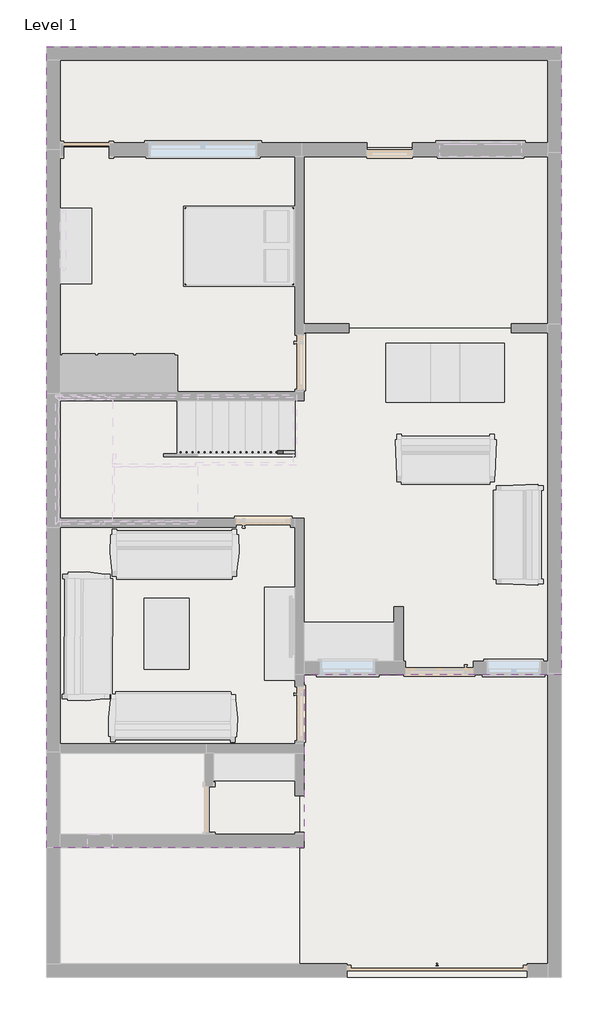
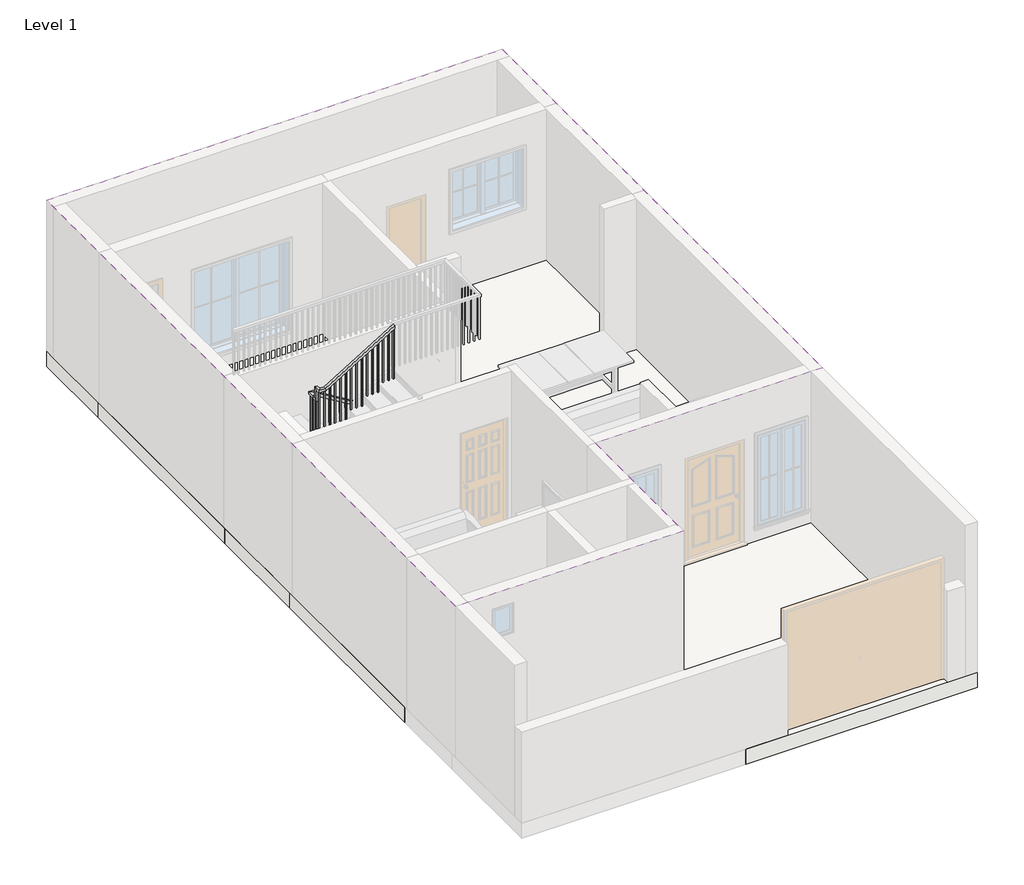
# One storey, part 2 of 3: 7 slabs, 1 covering, 1 railing.
"""IFC4 building model written with IfcOpenShell, lengths in millimetres."""

from ifc_helpers import new_model, si_unit, frame, origin, place, context, project, spatial, polyline, outline, extrude, faceted_brep, element, save

model = new_model("IFC4")

# Units and contexts
model_context = context("Model", 3, world=origin())
ifc_project = project(units=[si_unit("LENGTHUNIT", "METRE", prefix="MILLI")], contexts=[model_context])

# Site, building, storey
site = spatial("IfcSite", under=ifc_project)
building = spatial("IfcBuilding", under=site)
storey = spatial("IfcBuildingStorey", under=building, Name="Level 1", Elevation=0.0)

# Covering
placement = place(None, origin())
element("IfcCovering", 1, ObjectType="2' x 4' ACT System", at=placement, inside=storey, context=model_context, shape_type="SweptSolid", body=[
    extrude(outline(polyline([(3110.2994028, 8771.2870892), (3110.2994028, -1820.5129108), (-1233.1005972, -1820.5129108), (-1233.1005972, -4741.5129108), (-5576.5005972, -4741.5129108), (-5576.5005972, 8771.2870892), (3110.2994028, 8771.2870892)]), holes=[polyline([(-5347.9005972, 2802.2870892), (-5347.9005972, 821.0870892), (-3087.3005972, 821.0870892), (-3087.3005972, 1735.4870892), (-1233.1005972, 1735.4870892), (-1233.1005972, 2802.2870892), (-5347.9005972, 2802.2870892)])]), frame((0.0, 0.0, 3048.0), z_axis=(0.0, 0.0, 1.0), x_axis=(1.0, 0.0, 0.0)), (0.0, 0.0, 1.0), 57.15),
])

# Railing
element("IfcRailing", 2, ObjectType="Handrail - Rectangular", at=placement, inside=storey, context=model_context, shape_type="SolidModel", body=[
    faceted_brep([(-1385.5005972, 1905.095038, 1083.7333333), (-1385.5005972, 1905.095038, 1024.3318731), (-1385.5005972, 1955.895038, 1024.3318731), (-1385.5005972, 1955.895038, 1083.7333333), (-4382.7005972, 1905.095038, 2900.2181818), (-4433.5005972, 1905.095038, 2871.6046004), (-4433.5005972, 1955.895038, 2871.6046004), (-4382.7005972, 1955.895038, 2900.2181818), (-4382.7005972, 1905.095038, 2946.4), (-4433.5005972, 1905.095038, 2895.6), (-4433.5005972, 1955.895038, 2895.6), (-4382.7005972, 1955.895038, 2946.4), (-4458.9005972, 1905.095038, 2946.4), (-4458.9005972, 1905.095038, 2895.6), (-4509.7005972, 1955.895038, 2895.6), (-4509.7005972, 1955.895038, 2946.4), (-4458.9005972, 1828.895038, 2946.4), (-4458.9005972, 1828.895038, 2895.6), (-4509.7005972, 1828.895038, 2895.6), (-4509.7005972, 1828.895038, 2946.4), (-4458.9005972, 1760.8870892, 2946.4), (-4458.9005972, 1710.0870892, 2895.6), (-4509.7005972, 1710.0870892, 2895.6), (-4509.7005972, 1760.8870892, 2946.4), (-4458.9005972, 1760.8870892, 3161.9151515), (-4458.9005972, 1710.0870892, 3111.1151515), (-4509.7005972, 1710.0870892, 3111.1151515), (-4509.7005972, 1760.8870892, 3161.9151515), (-4458.9005972, 1684.6870892, 3161.9151515), (-4458.9005972, 1684.6870892, 3111.1151515), (-4509.7005972, 1633.8870892, 3111.1151515), (-4509.7005972, 1633.8870892, 3161.9151515), (-4382.7005972, 1684.6870892, 3161.9151515), (-4368.5081878, 1684.6870892, 3111.1151515), (-4368.5081878, 1633.8870892, 3111.1151515), (-4382.7005972, 1633.8870892, 3161.9151515), (-3061.9005972, 1684.6870892, 3962.4), (-3061.9005972, 1633.8870892, 3962.4), (-3061.9005972, 1633.8870892, 3902.9985397), (-3061.9005972, 1684.6870892, 3902.9985397)], [[[0, 1, 2, 3]], [[1, 0, 4, 5]], [[2, 1, 5, 6]], [[3, 2, 6, 7]], [[0, 3, 7, 4]], [[5, 4, 8, 9]], [[6, 5, 9, 10]], [[7, 6, 10, 11]], [[4, 7, 11, 8]], [[9, 8, 12, 13]], [[10, 9, 13, 14]], [[11, 10, 14, 15]], [[8, 11, 15, 12]], [[13, 12, 16, 17]], [[14, 13, 17, 18]], [[15, 14, 18, 19]], [[12, 15, 19, 16]], [[17, 16, 20, 21]], [[18, 17, 21, 22]], [[19, 18, 22, 23]], [[16, 19, 23, 20]], [[21, 20, 24, 25]], [[22, 21, 25, 26]], [[23, 22, 26, 27]], [[20, 23, 27, 24]], [[25, 24, 28, 29]], [[26, 25, 29, 30]], [[27, 26, 30, 31]], [[24, 27, 31, 28]], [[29, 28, 32, 33]], [[30, 29, 33, 34]], [[31, 30, 34, 35]], [[28, 31, 35, 32]], [[36, 37, 38, 39]], [[33, 32, 36, 39]], [[34, 33, 39, 38]], [[35, 34, 38, 37]], [[32, 35, 37, 36]]]),
    extrude(outline(polyline([(3835.6500549, -3173.0255972), (2878.6666667, -3173.0255972), (2878.6666667, -3153.9755972), (3847.1955094, -3153.9755972), (3835.6500549, -3173.0255972)])), frame((0.0, 1649.7620892, 0.0), z_axis=(0.0, 1.0, 0.0), x_axis=(0.0, 0.0, 1.0)), (0.0, 0.0, 1.0), 19.05),
    extrude(outline(polyline([(3774.0742973, -3274.6255972), (2878.6666667, -3274.6255972), (2878.6666667, -3255.5755972), (3785.6197519, -3255.5755972), (3774.0742973, -3274.6255972)])), frame((0.0, 1649.7620892, 0.0), z_axis=(0.0, 1.0, 0.0), x_axis=(0.0, 0.0, 1.0)), (0.0, 0.0, 1.0), 19.05),
    extrude(outline(polyline([(3712.4985397, -3376.2255972), (2709.3333333, -3376.2255972), (2709.3333333, -3357.1755972), (3724.0439943, -3357.1755972), (3712.4985397, -3376.2255972)])), frame((0.0, 1649.7620892, 0.0), z_axis=(0.0, 1.0, 0.0), x_axis=(0.0, 0.0, 1.0)), (0.0, 0.0, 1.0), 19.05),
    extrude(outline(polyline([(3650.9227822, -3477.8255972), (2709.3333333, -3477.8255972), (2709.3333333, -3458.7755972), (3662.4682367, -3458.7755972), (3650.9227822, -3477.8255972)])), frame((0.0, 1649.7620892, 0.0), z_axis=(0.0, 1.0, 0.0), x_axis=(0.0, 0.0, 1.0)), (0.0, 0.0, 1.0), 19.05),
    extrude(outline(polyline([(3589.3470246, -3579.4255972), (2709.3333333, -3579.4255972), (2709.3333333, -3560.3755972), (3600.8924791, -3560.3755972), (3589.3470246, -3579.4255972)])), frame((0.0, 1649.7620892, 0.0), z_axis=(0.0, 1.0, 0.0), x_axis=(0.0, 0.0, 1.0)), (0.0, 0.0, 1.0), 19.05),
    extrude(outline(polyline([(3527.771267, -3681.0255972), (2540.0, -3681.0255972), (2540.0, -3661.9755972), (3539.3167216, -3661.9755972), (3527.771267, -3681.0255972)])), frame((0.0, 1649.7620892, 0.0), z_axis=(0.0, 1.0, 0.0), x_axis=(0.0, 0.0, 1.0)), (0.0, 0.0, 1.0), 19.05),
    extrude(outline(polyline([(3466.1955094, -3782.6255972), (2540.0, -3782.6255972), (2540.0, -3763.5755972), (3477.740964, -3763.5755972), (3466.1955094, -3782.6255972)])), frame((0.0, 1649.7620892, 0.0), z_axis=(0.0, 1.0, 0.0), x_axis=(0.0, 0.0, 1.0)), (0.0, 0.0, 1.0), 19.05),
    extrude(outline(polyline([(3404.6197519, -3884.2255972), (2540.0, -3884.2255972), (2540.0, -3865.1755972), (3416.1652064, -3865.1755972), (3404.6197519, -3884.2255972)])), frame((0.0, 1649.7620892, 0.0), z_axis=(0.0, 1.0, 0.0), x_axis=(0.0, 0.0, 1.0)), (0.0, 0.0, 1.0), 19.05),
    extrude(outline(polyline([(3343.0439943, -3985.8255972), (2370.6666667, -3985.8255972), (2370.6666667, -3966.7755972), (3354.5894488, -3966.7755972), (3343.0439943, -3985.8255972)])), frame((0.0, 1649.7620892, 0.0), z_axis=(0.0, 1.0, 0.0), x_axis=(0.0, 0.0, 1.0)), (0.0, 0.0, 1.0), 19.05),
    extrude(outline(polyline([(3281.4682367, -4087.4255972), (2370.6666667, -4087.4255972), (2370.6666667, -4068.3755972), (3293.0136913, -4068.3755972), (3281.4682367, -4087.4255972)])), frame((0.0, 1649.7620892, 0.0), z_axis=(0.0, 1.0, 0.0), x_axis=(0.0, 0.0, 1.0)), (0.0, 0.0, 1.0), 19.05),
    extrude(outline(polyline([(3219.8924791, -4189.0255972), (2370.6666667, -4189.0255972), (2370.6666667, -4169.9755972), (3231.4379337, -4169.9755972), (3219.8924791, -4189.0255972)])), frame((0.0, 1649.7620892, 0.0), z_axis=(0.0, 1.0, 0.0), x_axis=(0.0, 0.0, 1.0)), (0.0, 0.0, 1.0), 19.05),
    extrude(outline(polyline([(3158.3167216, -4290.6255972), (2201.3333333, -4290.6255972), (2201.3333333, -4271.5755972), (3169.8621761, -4271.5755972), (3158.3167216, -4290.6255972)])), frame((0.0, 1649.7620892, 0.0), z_axis=(0.0, 1.0, 0.0), x_axis=(0.0, 0.0, 1.0)), (0.0, 0.0, 1.0), 19.05),
    extrude(outline(polyline([(3096.740964, -4392.2255972), (2201.3333333, -4392.2255972), (2201.3333333, -4373.1755972), (3108.2864185, -4373.1755972), (3096.740964, -4392.2255972)])), frame((0.0, 1649.7620892, 0.0), z_axis=(0.0, 1.0, 0.0), x_axis=(0.0, 0.0, 1.0)), (0.0, 0.0, 1.0), 19.05),
    extrude(outline(polyline([(-4474.7755972, 1736.820038), (-4474.7755972, 1717.770038), (-4493.8255972, 1717.770038), (-4493.8255972, 1736.820038), (-4474.7755972, 1736.820038)])), frame((0.0, 0.0, 2032.0), z_axis=(0.0, 0.0, 1.0), x_axis=(1.0, 0.0, 0.0)), (0.0, 0.0, 1.0), 1079.1151515),
    extrude(outline(polyline([(-4474.7755972, 1838.420038), (-4474.7755972, 1819.370038), (-4493.8255972, 1819.370038), (-4493.8255972, 1838.420038), (-4474.7755972, 1838.420038)])), frame((0.0, 0.0, 2032.0), z_axis=(0.0, 0.0, 1.0), x_axis=(1.0, 0.0, 0.0)), (0.0, 0.0, 1.0), 863.6),
    extrude(outline(polyline([(-4423.9755972, 1920.970038), (-4443.0255972, 1920.970038), (-4443.0255972, 1940.020038), (-4423.9755972, 1940.020038), (-4423.9755972, 1920.970038)])), frame((0.0, 0.0, 1862.6666667), z_axis=(0.0, 0.0, 1.0), x_axis=(1.0, 0.0, 0.0)), (0.0, 0.0, 1.0), 1032.9333333),
    extrude(outline(polyline([(2815.80157, -4341.4255972), (1862.6666667, -4341.4255972), (1862.6666667, -4322.3755972), (2804.2561155, -4322.3755972), (2815.80157, -4341.4255972)])), frame((0.0, 1920.970038, 0.0), z_axis=(0.0, 1.0, 0.0), x_axis=(0.0, 0.0, 1.0)), (0.0, 0.0, 1.0), 19.05),
    extrude(outline(polyline([(2754.2258125, -4239.8255972), (1862.6666667, -4239.8255972), (1862.6666667, -4220.7755972), (2742.6803579, -4220.7755972), (2754.2258125, -4239.8255972)])), frame((0.0, 1920.970038, 0.0), z_axis=(0.0, 1.0, 0.0), x_axis=(0.0, 0.0, 1.0)), (0.0, 0.0, 1.0), 19.05),
    extrude(outline(polyline([(2692.6500549, -4138.2255972), (1693.3333333, -4138.2255972), (1693.3333333, -4119.1755972), (2681.1046004, -4119.1755972), (2692.6500549, -4138.2255972)])), frame((0.0, 1920.970038, 0.0), z_axis=(0.0, 1.0, 0.0), x_axis=(0.0, 0.0, 1.0)), (0.0, 0.0, 1.0), 19.05),
    extrude(outline(polyline([(2631.0742973, -4036.6255972), (1693.3333333, -4036.6255972), (1693.3333333, -4017.5755972), (2619.5288428, -4017.5755972), (2631.0742973, -4036.6255972)])), frame((0.0, 1920.970038, 0.0), z_axis=(0.0, 1.0, 0.0), x_axis=(0.0, 0.0, 1.0)), (0.0, 0.0, 1.0), 19.05),
    extrude(outline(polyline([(2569.4985397, -3935.0255972), (1693.3333333, -3935.0255972), (1693.3333333, -3915.9755972), (2557.9530852, -3915.9755972), (2569.4985397, -3935.0255972)])), frame((0.0, 1920.970038, 0.0), z_axis=(0.0, 1.0, 0.0), x_axis=(0.0, 0.0, 1.0)), (0.0, 0.0, 1.0), 19.05),
    extrude(outline(polyline([(2507.9227822, -3833.4255972), (1524.0, -3833.4255972), (1524.0, -3814.3755972), (2496.3773276, -3814.3755972), (2507.9227822, -3833.4255972)])), frame((0.0, 1920.970038, 0.0), z_axis=(0.0, 1.0, 0.0), x_axis=(0.0, 0.0, 1.0)), (0.0, 0.0, 1.0), 19.05),
    extrude(outline(polyline([(2446.3470246, -3731.8255972), (1524.0, -3731.8255972), (1524.0, -3712.7755972), (2434.80157, -3712.7755972), (2446.3470246, -3731.8255972)])), frame((0.0, 1920.970038, 0.0), z_axis=(0.0, 1.0, 0.0), x_axis=(0.0, 0.0, 1.0)), (0.0, 0.0, 1.0), 19.05),
    extrude(outline(polyline([(2384.771267, -3630.2255972), (1524.0, -3630.2255972), (1524.0, -3611.1755972), (2373.2258125, -3611.1755972), (2384.771267, -3630.2255972)])), frame((0.0, 1920.970038, 0.0), z_axis=(0.0, 1.0, 0.0), x_axis=(0.0, 0.0, 1.0)), (0.0, 0.0, 1.0), 19.05),
    extrude(outline(polyline([(2323.1955094, -3528.6255972), (1354.6666667, -3528.6255972), (1354.6666667, -3509.5755972), (2311.6500549, -3509.5755972), (2323.1955094, -3528.6255972)])), frame((0.0, 1920.970038, 0.0), z_axis=(0.0, 1.0, 0.0), x_axis=(0.0, 0.0, 1.0)), (0.0, 0.0, 1.0), 19.05),
    extrude(outline(polyline([(2261.6197519, -3427.0255972), (1354.6666667, -3427.0255972), (1354.6666667, -3407.9755972), (2250.0742973, -3407.9755972), (2261.6197519, -3427.0255972)])), frame((0.0, 1920.970038, 0.0), z_axis=(0.0, 1.0, 0.0), x_axis=(0.0, 0.0, 1.0)), (0.0, 0.0, 1.0), 19.05),
    extrude(outline(polyline([(2200.0439943, -3325.4255972), (1185.3333333, -3325.4255972), (1185.3333333, -3306.3755972), (2188.4985397, -3306.3755972), (2200.0439943, -3325.4255972)])), frame((0.0, 1920.970038, 0.0), z_axis=(0.0, 1.0, 0.0), x_axis=(0.0, 0.0, 1.0)), (0.0, 0.0, 1.0), 19.05),
    extrude(outline(polyline([(2138.4682367, -3223.8255972), (1185.3333333, -3223.8255972), (1185.3333333, -3204.7755972), (2126.9227822, -3204.7755972), (2138.4682367, -3223.8255972)])), frame((0.0, 1920.970038, 0.0), z_axis=(0.0, 1.0, 0.0), x_axis=(0.0, 0.0, 1.0)), (0.0, 0.0, 1.0), 19.05),
    extrude(outline(polyline([(2076.8924791, -3122.2255972), (1185.3333333, -3122.2255972), (1185.3333333, -3103.1755972), (2065.3470246, -3103.1755972), (2076.8924791, -3122.2255972)])), frame((0.0, 1920.970038, 0.0), z_axis=(0.0, 1.0, 0.0), x_axis=(0.0, 0.0, 1.0)), (0.0, 0.0, 1.0), 19.05),
    extrude(outline(polyline([(2015.3167216, -3020.6255972), (1016.0, -3020.6255972), (1016.0, -3001.5755972), (2003.771267, -3001.5755972), (2015.3167216, -3020.6255972)])), frame((0.0, 1920.970038, 0.0), z_axis=(0.0, 1.0, 0.0), x_axis=(0.0, 0.0, 1.0)), (0.0, 0.0, 1.0), 19.05),
    extrude(outline(polyline([(1953.740964, -2919.0255972), (1016.0, -2919.0255972), (1016.0, -2899.9755972), (1942.1955094, -2899.9755972), (1953.740964, -2919.0255972)])), frame((0.0, 1920.970038, 0.0), z_axis=(0.0, 1.0, 0.0), x_axis=(0.0, 0.0, 1.0)), (0.0, 0.0, 1.0), 19.05),
    extrude(outline(polyline([(1892.1652064, -2817.4255972), (1016.0, -2817.4255972), (1016.0, -2798.3755972), (1880.6197519, -2798.3755972), (1892.1652064, -2817.4255972)])), frame((0.0, 1920.970038, 0.0), z_axis=(0.0, 1.0, 0.0), x_axis=(0.0, 0.0, 1.0)), (0.0, 0.0, 1.0), 19.05),
    extrude(outline(polyline([(1830.5894488, -2715.8255972), (846.6666667, -2715.8255972), (846.6666667, -2696.7755972), (1819.0439943, -2696.7755972), (1830.5894488, -2715.8255972)])), frame((0.0, 1920.970038, 0.0), z_axis=(0.0, 1.0, 0.0), x_axis=(0.0, 0.0, 1.0)), (0.0, 0.0, 1.0), 19.05),
    extrude(outline(polyline([(1769.0136913, -2614.2255972), (846.6666667, -2614.2255972), (846.6666667, -2595.1755972), (1757.4682367, -2595.1755972), (1769.0136913, -2614.2255972)])), frame((0.0, 1920.970038, 0.0), z_axis=(0.0, 1.0, 0.0), x_axis=(0.0, 0.0, 1.0)), (0.0, 0.0, 1.0), 19.05),
    extrude(outline(polyline([(1707.4379337, -2512.6255972), (846.6666667, -2512.6255972), (846.6666667, -2493.5755972), (1695.8924791, -2493.5755972), (1707.4379337, -2512.6255972)])), frame((0.0, 1920.970038, 0.0), z_axis=(0.0, 1.0, 0.0), x_axis=(0.0, 0.0, 1.0)), (0.0, 0.0, 1.0), 19.05),
    extrude(outline(polyline([(1645.8621761, -2411.0255972), (677.3333333, -2411.0255972), (677.3333333, -2391.9755972), (1634.3167216, -2391.9755972), (1645.8621761, -2411.0255972)])), frame((0.0, 1920.970038, 0.0), z_axis=(0.0, 1.0, 0.0), x_axis=(0.0, 0.0, 1.0)), (0.0, 0.0, 1.0), 19.05),
    extrude(outline(polyline([(1584.2864185, -2309.4255972), (677.3333333, -2309.4255972), (677.3333333, -2290.3755972), (1572.740964, -2290.3755972), (1584.2864185, -2309.4255972)])), frame((0.0, 1920.970038, 0.0), z_axis=(0.0, 1.0, 0.0), x_axis=(0.0, 0.0, 1.0)), (0.0, 0.0, 1.0), 19.05),
    extrude(outline(polyline([(1522.710661, -2207.8255972), (508.0, -2207.8255972), (508.0, -2188.7755972), (1511.1652064, -2188.7755972), (1522.710661, -2207.8255972)])), frame((0.0, 1920.970038, 0.0), z_axis=(0.0, 1.0, 0.0), x_axis=(0.0, 0.0, 1.0)), (0.0, 0.0, 1.0), 19.05),
    extrude(outline(polyline([(1461.1349034, -2106.2255972), (508.0, -2106.2255972), (508.0, -2087.1755972), (1449.5894488, -2087.1755972), (1461.1349034, -2106.2255972)])), frame((0.0, 1920.970038, 0.0), z_axis=(0.0, 1.0, 0.0), x_axis=(0.0, 0.0, 1.0)), (0.0, 0.0, 1.0), 19.05),
    extrude(outline(polyline([(1399.5591458, -2004.6255972), (508.0, -2004.6255972), (508.0, -1985.5755972), (1388.0136913, -1985.5755972), (1399.5591458, -2004.6255972)])), frame((0.0, 1920.970038, 0.0), z_axis=(0.0, 1.0, 0.0), x_axis=(0.0, 0.0, 1.0)), (0.0, 0.0, 1.0), 19.05),
    extrude(outline(polyline([(1337.9833882, -1903.0255972), (338.6666667, -1903.0255972), (338.6666667, -1883.9755972), (1326.4379337, -1883.9755972), (1337.9833882, -1903.0255972)])), frame((0.0, 1920.970038, 0.0), z_axis=(0.0, 1.0, 0.0), x_axis=(0.0, 0.0, 1.0)), (0.0, 0.0, 1.0), 19.05),
    extrude(outline(polyline([(1276.4076307, -1801.4255972), (338.6666667, -1801.4255972), (338.6666667, -1782.3755972), (1264.8621761, -1782.3755972), (1276.4076307, -1801.4255972)])), frame((0.0, 1920.970038, 0.0), z_axis=(0.0, 1.0, 0.0), x_axis=(0.0, 0.0, 1.0)), (0.0, 0.0, 1.0), 19.05),
    extrude(outline(polyline([(1214.8318731, -1699.8255972), (338.6666667, -1699.8255972), (338.6666667, -1680.7755972), (1203.2864185, -1680.7755972), (1214.8318731, -1699.8255972)])), frame((0.0, 1920.970038, 0.0), z_axis=(0.0, 1.0, 0.0), x_axis=(0.0, 0.0, 1.0)), (0.0, 0.0, 1.0), 19.05),
    extrude(outline(polyline([(1153.2561155, -1598.2255972), (169.3333333, -1598.2255972), (169.3333333, -1579.1755972), (1141.710661, -1579.1755972), (1153.2561155, -1598.2255972)])), frame((0.0, 1920.970038, 0.0), z_axis=(0.0, 1.0, 0.0), x_axis=(0.0, 0.0, 1.0)), (0.0, 0.0, 1.0), 19.05),
    extrude(outline(polyline([(1091.6803579, -1496.6255972), (169.3333333, -1496.6255972), (169.3333333, -1477.5755972), (1080.1349034, -1477.5755972), (1091.6803579, -1496.6255972)])), frame((0.0, 1920.970038, 0.0), z_axis=(0.0, 1.0, 0.0), x_axis=(0.0, 0.0, 1.0)), (0.0, 0.0, 1.0), 19.05),
    extrude(outline(polyline([(-4474.7755972, 1668.8120892), (-4474.7755972, 1649.7620892), (-4493.8255972, 1649.7620892), (-4493.8255972, 1668.8120892), (-4474.7755972, 1668.8120892)])), frame((0.0, 0.0, 2032.0), z_axis=(0.0, 0.0, 1.0), x_axis=(1.0, 0.0, 0.0)), (0.0, 0.0, 1.0), 1079.1151515),
    extrude(outline(polyline([(-4474.7755972, 1920.970038), (-4493.8255972, 1920.970038), (-4493.8255972, 1940.020038), (-4474.7755972, 1940.020038), (-4474.7755972, 1920.970038)])), frame((0.0, 0.0, 2032.0), z_axis=(0.0, 0.0, 1.0), x_axis=(1.0, 0.0, 0.0)), (0.0, 0.0, 1.0), 863.6),
    extrude(outline(polyline([(3891.4530852, -3080.9505972), (2878.6666667, -3080.9505972), (2878.6666667, -3061.9005972), (3902.9985397, -3061.9005972), (3891.4530852, -3080.9505972)])), frame((0.0, 1649.7620892, 0.0), z_axis=(0.0, 1.0, 0.0), x_axis=(0.0, 0.0, 1.0)), (0.0, 0.0, 1.0), 19.05),
    extrude(outline(polyline([(1035.8773276, -1404.5505972), (169.3333333, -1404.5505972), (169.3333333, -1385.5005972), (1024.3318731, -1385.5005972), (1035.8773276, -1404.5505972)])), frame((0.0, 1920.970038, 0.0), z_axis=(0.0, 1.0, 0.0), x_axis=(0.0, 0.0, 1.0)), (0.0, 0.0, 1.0), 19.05),
])

# Slabs
element("IfcSlab", 3, ObjectType="Generic - 12\"", at=placement, inside=storey, context=model_context, shape_type="SweptSolid", body=[
    extrude(outline(polyline([(3110.2994028, 8771.2870892), (3110.2994028, 7069.4870892), (-5576.5005972, 7069.4870892), (-5576.5005972, 8771.2870892), (3110.2994028, 8771.2870892)])), frame((0.0, 0.0, -304.8), z_axis=(0.0, 0.0, 1.0), x_axis=(1.0, 0.0, 0.0)), (0.0, 0.0, 1.0), 304.8),
])
element("IfcSlab", 4, ObjectType="Generic - 12\"", at=placement, inside=storey, context=model_context, shape_type="SweptSolid", body=[
    extrude(outline(polyline([(-1309.3005972, 7069.4870892), (-1309.3005972, 2878.4870892), (-5576.5005972, 2878.4870892), (-5576.5005972, 7069.4870892), (-1309.3005972, 7069.4870892)])), frame((0.0, 0.0, -304.8), z_axis=(0.0, 0.0, 1.0), x_axis=(1.0, 0.0, 0.0)), (0.0, 0.0, 1.0), 304.8),
])
element("IfcSlab", 5, ObjectType="Generic - 12\"", at=placement, inside=storey, context=model_context, shape_type="SweptSolid", body=[
    extrude(outline(polyline([(-1309.3005972, 4021.4870892), (-1309.3005972, 7069.4870892), (3110.2994028, 7069.4870892), (3110.2994028, 4021.4870892), (-1309.3005972, 4021.4870892)])), frame((0.0, 0.0, -304.8), z_axis=(0.0, 0.0, 1.0), x_axis=(1.0, 0.0, 0.0)), (0.0, 0.0, 1.0), 304.8),
])
element("IfcSlab", 6, ObjectType="Generic - 12\"", at=placement, inside=storey, context=model_context, shape_type="SweptSolid", body=[
    extrude(outline(polyline([(-5576.5005972, 2878.4870892), (-1309.3005972, 2878.4870892), (-1309.3005972, 4021.4870892), (3110.2994028, 4021.4870892), (3110.2994028, -1706.2129108), (-1233.1005972, -1706.2129108), (-1233.1005972, 744.8870892), (-5576.5005972, 744.8870892), (-5576.5005972, 2878.4870892)])), frame((0.0, 0.0, -304.8), z_axis=(0.0, 0.0, 1.0), x_axis=(1.0, 0.0, 0.0)), (0.0, 0.0, 1.0), 304.8),
])
element("IfcSlab", 7, ObjectType="Generic - 12\"", at=placement, inside=storey, context=model_context, shape_type="SweptSolid", body=[
    extrude(outline(polyline([(-1309.3005972, 744.8870892), (-1309.3005972, -3065.1129108), (-5576.5005972, -3065.1129108), (-5576.5005972, 744.8870892), (-1309.3005972, 744.8870892)])), frame((0.0, 0.0, -304.8), z_axis=(0.0, 0.0, 1.0), x_axis=(1.0, 0.0, 0.0)), (0.0, 0.0, 1.0), 304.8),
])
element("IfcSlab", 8, ObjectType="Generic - 12\"", at=placement, inside=storey, context=model_context, shape_type="SweptSolid", body=[
    extrude(outline(polyline([(-2833.3005972, -4627.2129108), (-2833.3005972, -3065.1129108), (-1309.3005972, -3065.1129108), (-1309.3005972, -4627.2129108), (-2833.3005972, -4627.2129108)])), frame((0.0, 0.0, -304.8), z_axis=(0.0, 0.0, 1.0), x_axis=(1.0, 0.0, 0.0)), (0.0, 0.0, 1.0), 304.8),
])
element("IfcSlab", 9, ObjectType="Generic - 12\"", at=placement, inside=storey, context=model_context, shape_type="SweptSolid", body=[
    extrude(outline(polyline([(3110.2994028, -1706.2129108), (3110.2994028, -6925.9129108), (-1309.3005972, -6925.9129108), (-1309.3005972, -1706.2129108), (3110.2994028, -1706.2129108)])), frame((0.0, 0.0, -304.8), z_axis=(0.0, 0.0, 1.0), x_axis=(1.0, 0.0, 0.0)), (0.0, 0.0, 1.0), 304.8),
])

save(model, "model.ifc")

# Revit data of these elements
# Type "2' x 4' ACT System"
#   Assembly Code = "C3030210"
#   built-in parameter 1002203 = 1 (stored number, unit not read)
#   built-in parameter 1002202 = 1 (stored number, unit not read)
#   Layers, outside or top first: 0' - 1 5/8" "Default" (function 1); 0' - 0 5/8" "Acoustic Ceiling Tile 24 x 48" (function 5)
# Type "Handrail - Rectangular"
#   Assembly Code = "C2010400"
#   built-in parameter 1008612 = 0.0416667 (stored number, unit not read)
#   built-in parameter 1008611 = 0.0416667 (stored number, unit not read)
#   built-in parameter 1008609 = 0.333333 (stored number, unit not read)
#   built-in parameter 1008604 = 0.166667 (stored number, unit not read)
#   built-in parameter 1008603 = 0.166667 (stored number, unit not read)
#   Railing Height = 3' - 0"
#   built-in parameter 1008630 = 2
#   built-in parameter 1008610 = 2
#   built-in parameter 1008618 = Baluster - Square : 3/4"
# Type "Generic - 12\""
#   Assembly Code = "B1010"
#   Function = 0
#   Layers, outside or top first: 1' - 0" no material (function 1)
# Element 1 (IfcCovering, "2' x 4' ACT System")
#   Height Offset From Level = 10' - 0"
#   Phase Created = New Construction
#   Materials on its faces: "Acoustic Ceiling Tile 24 x 48", "Vinyl Composition Tile"
# Element 2 (IfcRailing, "Handrail - Rectangular")
#   Phase Created = New Construction
# Element 3 (IfcSlab, "Generic - 12\"")
#   Height Offset From Level = 0' - 0"
#   Phase Created = New Construction
#   Materials on its faces: "Brick, Common", "Wood - Stained", "Default Floor", "FRONT WALL"
# Element 4 (IfcSlab, "Generic - 12\"")
#   Height Offset From Level = 0' - 0"
#   Phase Created = New Construction
#   Materials on its faces: "Default Floor", "FLOOR HALL", "FRONT WALL"
# Element 5 (IfcSlab, "Generic - 12\"")
#   built-in parameter 1001955 = -1.5708 (stored number, unit not read)
#   Height Offset From Level = 0' - 0"
#   Phase Created = New Construction
#   Materials on its faces: "Default Floor", "FLOOR HALL", "Brick, Common"
# Element 6 (IfcSlab, "Generic - 12\"")
#   built-in parameter 1001955 = 3.14159 (stored number, unit not read)
#   Height Offset From Level = 0' - 0"
#   Phase Created = New Construction
#   Materials on its faces: "Default Floor", "FLOOR HALL", "Brick, Common", "FRONT WALL"
# Element 7 (IfcSlab, "Generic - 12\"")
#   Height Offset From Level = 0' - 0"
#   Phase Created = New Construction
#   Materials on its faces: "Default Floor", "FRONT WALL", "FLOOR HALL"
# Element 8 (IfcSlab, "Generic - 12\"")
#   built-in parameter 1001955 = -1.5708 (stored number, unit not read)
#   Height Offset From Level = 0' - 0"
#   Phase Created = New Construction
#   Materials on its faces: "Default Floor", "Wood Planks"
# Element 9 (IfcSlab, "Generic - 12\"")
#   Height Offset From Level = 0' - 0"
#   Phase Created = New Construction
#   Materials on its faces: "Default Floor", "WALL 1", "Brick, Common", "FRONT WALL"
# Materials
#   "Default": colour RGB 127 127 127, transparency 0, Cost = 0
#   "Acoustic Ceiling Tile 24 x 48": class "Generic", colour RGB 229 229 229, transparency 0, Description = "Acoustic Ceiling Tile 24 x 48", Cost = 0
#   "Vinyl Composition Tile": class "Generic", colour RGB 179 160 124, transparency 0, Description = "Vinyl Composition Tile", Cost = 0
#   "Brick, Common": class "Masonry", colour RGB 170 98 104, transparency 0, Description = "Common brick", Cost = 0
#   "Wood - Stained": class "Wood", colour RGB 224 178 126, transparency 0, Cost = 0
#   "Default Floor": colour RGB 128 128 128, transparency 0, Cost = 0
#   "FRONT WALL": class "Generic", colour RGB 120 120 120, transparency 0, Cost = 0
#   "FLOOR HALL": class "Generic", colour RGB 120 120 120, transparency 0, Cost = 0
#   "Wood Planks": class "Wood", colour RGB 193 160 115, transparency 0, Description = "Physical material.", Cost = 0
#   "WALL 1": class "Generic", colour RGB 120 120 120, transparency 0, Cost = 0
